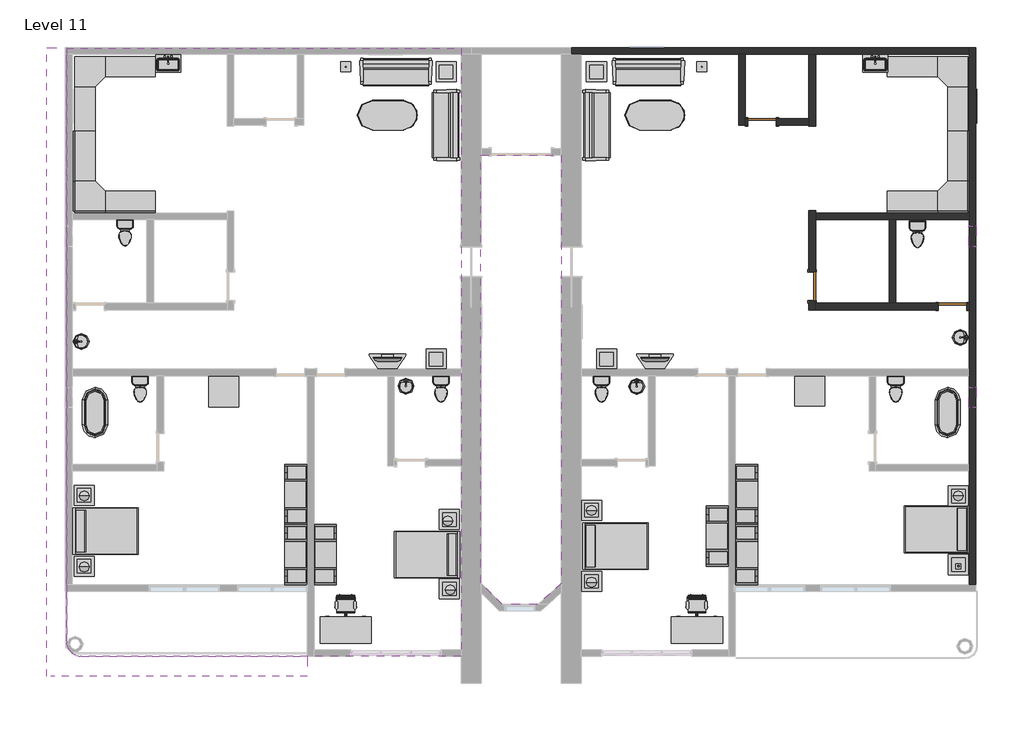
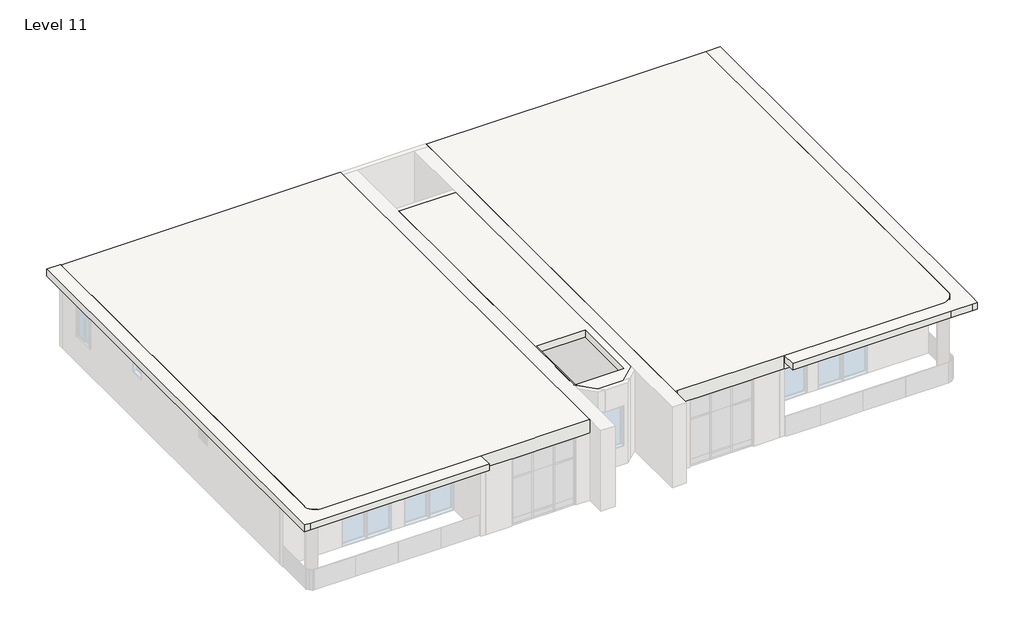
# One storey, part 3 of 3: 42 furniture elements, 14 flow terminals, 10 light fixtures, 9 walls, 3 doors, 3 slabs, 3 windows.
# Revit data of these elements (continued)
# Elements 40, 41 (IfcFurniture, "TV Stand : TV Stand") (continued)
#   Phase Created = New Construction
#   Materials on its faces: "Melamine - Gray", "Glass - Shelves"
# Elements 42, 43, 44, 45, 46, 47, 48, 49, 50, 51, 52, 53 (IfcFurniture, "Table-Coffee : 24\" x 24\" x 24\"")
#   Phase Created = New Construction
#   Materials on its faces: "Glass - Clear, Grey"
# Elements 54, 55 (IfcFurniture, "Table-Dining Oval : 36\" x 72\"")
#   Phase Created = New Construction
#   Materials on its faces: "Steel, Chrome Plated", "Glass - Clear, Grey"
# Elements 56, 57 (IfcFurniture, "Table-Rectangular : 36\" x 36\"")
#   Phase Created = New Construction
#   Materials on its faces: "Birch"
# Elements 58, 59 (IfcFurniture, "Work Station Cubicle : 96\" x 96\"")
#   Phase Created = New Construction
#   Materials on its faces: "Textile - Light Gray", "Laminate, Ivory, Matte"
# Element 60 (IfcLightFixture, "100W - 120V")
#   Mark = "124"
#   Phase Created = New Construction
#   Materials on its faces: "Steel, Chrome Plated", "Glass, Frosted"
# Element 61 (IfcLightFixture, "100W - 120V")
#   Mark = "125"
#   Phase Created = New Construction
#   Materials on its faces: "Steel, Chrome Plated", "Glass, Frosted"
# Element 62 (IfcLightFixture, "Table Lamp - Hemispheric : 60W - 120V")
#   Mark = "126"
#   Phase Created = New Construction
#   Materials on its faces: "Steel, Chrome Plated", "Glass, Frosted", "Birch"
# Element 63 (IfcLightFixture, "Table Lamp - Hemispheric : 60W - 120V")
#   Mark = "127"
#   Phase Created = New Construction
#   Materials on its faces: "Steel, Chrome Plated", "Glass, Frosted", "Birch"
# Element 64 (IfcLightFixture, "Table Lamp - Hemispheric : 60W - 120V")
#   Mark = "128"
#   Phase Created = New Construction
#   Materials on its faces: "Steel, Chrome Plated", "Glass, Frosted", "Birch"
# Element 65 (IfcLightFixture, "Table Lamp - Hemispheric : 60W - 120V")
#   Mark = "129"
#   Phase Created = New Construction
#   Materials on its faces: "Steel, Chrome Plated", "Glass, Frosted", "Birch"
# Element 66 (IfcLightFixture, "Table Lamp - Hemispheric : 60W - 120V")
#   Mark = "130"
#   Phase Created = New Construction
#   Materials on its faces: "Steel, Chrome Plated", "Glass, Frosted", "Birch"
# Element 67 (IfcLightFixture, "Table Lamp - Hemispheric : 60W - 120V")
#   Mark = "131"
#   Phase Created = New Construction
#   Materials on its faces: "Steel, Chrome Plated", "Glass, Frosted", "Birch"
# Element 68 (IfcLightFixture, "Table Lamp - Hemispheric : 60W - 120V")
#   Mark = "132"
#   Phase Created = New Construction
#   Materials on its faces: "Steel, Chrome Plated", "Glass, Frosted", "Birch"
# Element 69 (IfcLightFixture, "Table Lamp - Hemispheric : 60W - 120V")
#   Mark = "133"
#   Phase Created = New Construction
#   Materials on its faces: "Steel, Chrome Plated", "Glass, Frosted", "Birch"
# Element 70 (IfcSlab, "Generic - 12\" cream")
#   Height Offset From Level = 12' - 0"
#   Phase Created = New Construction
#   Materials on its faces: "Parking Stripe"
# Element 71 (IfcSlab, "Generic - 12\" white")
#   built-in parameter 1001955 = 3.14159 (stored number, unit not read)
#   Height Offset From Level = 12' - 0"
#   Phase Created = New Construction
#   Materials on its faces: "Door - Frame"
# Element 72 (IfcSlab, "Generic - 12\" white")
#   Height Offset From Level = 12' - 0"
#   Phase Created = New Construction
#   Materials on its faces: "Door - Frame"
# Elements 73, 74, 75, 76, 77, 78, 79, 80 (IfcWall, "Generic - 8\" cream")
#   Top Offset = 0' - 0"
#   Base Offset = 0' - 0"
#   Unconnected Height = 10' - 0"
#   wall height = 10' - 0"
#   Phase Created = New Construction
#   Base Constraint = Level 11
#   Materials on its faces: "Parking Stripe"
# Element 81 (IfcWall, "Generic - 8\" white")
#   Top Offset = 0' - 0"
#   Base Offset = 0' - 0"
#   Unconnected Height = 10' - 0"
#   wall height = 10' - 0"
#   Phase Created = New Construction
#   Base Constraint = Level 11
#   Materials on its faces: "Door - Frame", "Parking Stripe"
# Element 82 (IfcWindow, "Louvers with Trim : 24\" x 24\"")
#   Mark = "243"
#   Phase Created = New Construction
#   Materials on its faces: "Glass", "Iron, Ductile"
# Element 83 (IfcWindow, "Louvers with Trim : 24\" x 24\"")
#   Mark = "244"
#   Phase Created = New Construction
#   Materials on its faces: "Glass", "Iron, Ductile"
# Element 84 (IfcWindow, "Slider with Trim : 36\" x 48\"")
#   Mark = "240"
#   Phase Created = New Construction
#   Materials on its faces: "Iron, Ductile", "Glass"
# Materials
#   "Wood - Birch - Solid Stained Light Low Gloss": class "Wood", colour RGB 210 159 95, transparency 0, Cost = 0
#   "Paint - Sienna": colour RGB 118 70 51, transparency 0, Cost = 0
#   "Steel, Polished": class "Metal", colour RGB 57 57 57, transparency 0, Description = "Polished steel", Cost = 0
#   "Porcelain, Linen": class "Ceramic", colour RGB 249 239 230, transparency 0, Description = "Porcelain, linen", Cost = 0
#   "Laminate, Linen, Matte": class "Plastic", colour RGB 249 239 230, transparency 0, Description = "Plastic Laminate - Linen, Matte", Cost = 0
#   "Porcelain, Ivory": class "Ceramic", colour RGB 247 247 239, transparency 0, Description = "Porcelain, ivory", Cost = 0
#   "Laminate, Ivory, Matte": class "Plastic", colour RGB 247 247 239, transparency 0, Description = "Plastic Laminate - Ivory, Matte", Cost = 0
#   "Birch": class "Wood", colour RGB 224 178 126, transparency 0, Description = "Betula Alleghaniensis", Cost = 0
#   "Linen, White": class "Textile", colour RGB 247 247 239, transparency 0, Description = "Linen, white", Cost = 0
#   "Plastic, Opaque Black": class "Plastic", colour RGB 0 0 0, transparency 0.7, Description = "Plastic, generic, opaque black", Cost = 0
#   "Textile - Slate Blue": class "Fabric", colour RGB 98 102 118, transparency 0
#   "Steel, Chrome Plated": class "Metal", colour RGB 17 17 17, transparency 0, Description = "Chromiuim plated steel", Cost = 0
#   "Cherry": class "Wood", colour RGB 226 177 128, transparency 0, Description = "Prunus Serotina", Cost = 0
#   "Linen, Beige": class "Textile", colour RGB 249 239 230, transparency 0, Description = "Linen, beige", Cost = 0
#   "Melamine - Gray": class "Wood", colour RGB 49 49 49, transparency 0
#   "Glass - Clear, Grey": class "Glass", colour RGB 252 255 255, transparency 0.64
#   "Textile - Light Gray": class "Fabric", colour RGB 204 204 204, transparency 0
#   "Glass, Frosted": class "Glass", colour RGB 250 244 225, transparency 0.55, Description = "physical material", Cost = 0
#   "Parking Stripe": class "Paint", colour RGB 250 250 91, transparency 0, Cost = 0
#   "Door - Frame": colour RGB 118 70 51, transparency 0, Cost = 0
#   "Iron, Ductile": class "Metal", colour RGB 0 0 0, transparency 0, Description = "Ductile cast iron", Cost = 0
#   "Glass": class "Glass", colour RGB 0 128 192, transparency 0.75, Description = "Soda Lime Glass", Cost = 0
#   "TV - Black": colour RGB 49 49 49, transparency 0
#   "TV - Glass": colour RGB 157 157 157, transparency 0.9
#   "TV - Screen": colour RGB 0 0 0, transparency 0
#   "Glass - Shelves": class "Glass", colour RGB 167 167 167, transparency 0.9
